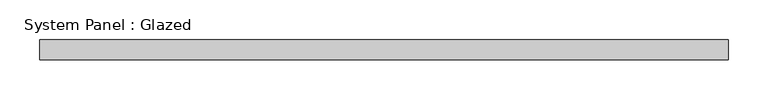
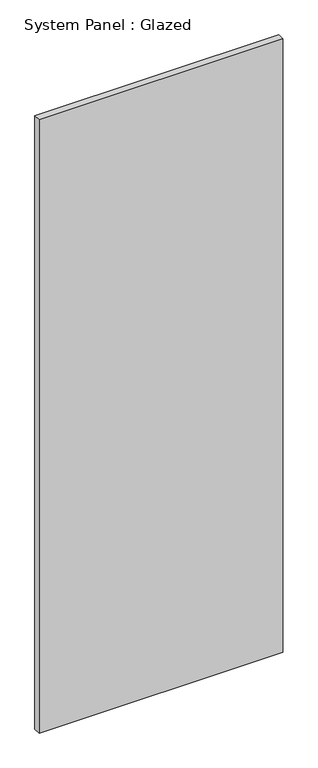
"""IFC4 building model written with IfcOpenShell, lengths in millimetres: plate geometry, System Panel : Glazed."""

from ifc_helpers import new_model, si_unit, origin, origin_with_axes, place, context, project, spatial, polyline, outline, extrude, source, transform, mapped, element, save


def system_panel_glazed_12377b85(model_context):
    return source(origin(), model_context, "Body", "SweptSolid", [
        extrude(outline(polyline([(434.975, 19.05), (-434.975, 19.05), (-434.975, 44.45), (434.975, 44.45), (434.975, 19.05)])), origin_with_axes(), (0.0, 0.0, 1.0), 2313.0217298),
    ])


if __name__ == "__main__":
    model = new_model("IFC4")
    model_context = context("Model", 3, world=origin())
    ifc_project = project(units=[si_unit("LENGTHUNIT", "METRE", prefix="MILLI")], contexts=[model_context])
    site = spatial("IfcSite", under=ifc_project)
    building = spatial("IfcBuilding", under=site)
    placement = place(None, origin())
    system_panel_glazed_shape = system_panel_glazed_12377b85(model_context)
    element("IfcPlate", 1, ObjectType="System Panel : Glazed", at=placement, inside=building, context=model_context, shape_type="MappedRepresentation", body=[
        mapped(system_panel_glazed_shape, transform((0.0, 0.0, 0.0), x_axis=(1.0, 0.0, 0.0), y_axis=(0.0, 1.0, 0.0), z_axis=(0.0, 0.0, 1.0))),
    ])
    save(model, "model.ifc")

# Revit data of these elements
# Type "System Panel : Glazed"
#   Construction Type Id = "GSP4R"
#   Analytic Construction = "1/8 in Pilkington single glazing"
#   Visual Light Transmittance = 0.9
#   Solar Heat Gain Coefficient = 0.86
#   Heat Transfer Coefficient (U) = 1.18115 BTU/(h·ft²·°F)
#   Define Thermal Properties by = 1
# Element 1 (IfcPlate, "System Panel : Glazed")
#   Materials on its faces: "Glass"
# Materials
#   "Glass": class "Glass", colour RGB 0 128 192, transparency 0.75, Description = "Soda Lime Glass", Cost = 0
